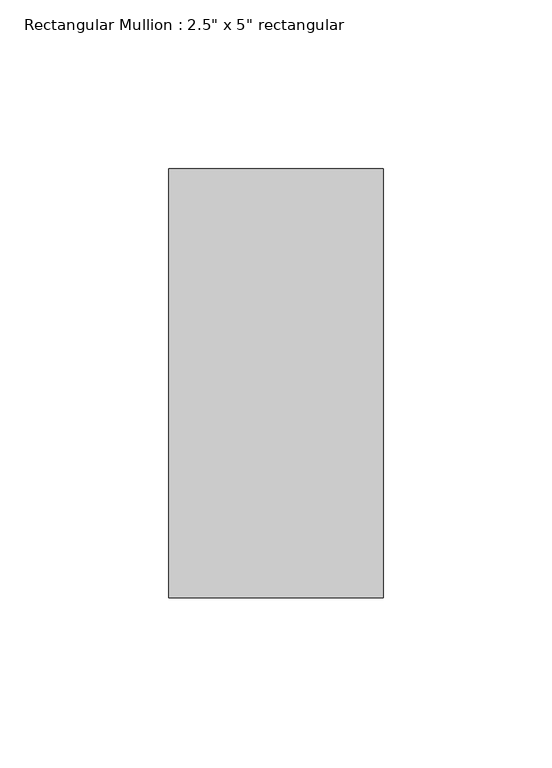
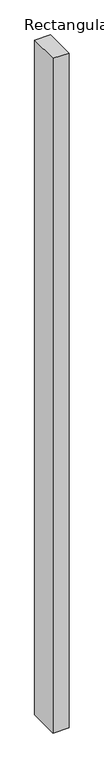
"""IFC4 building model written with IfcOpenShell, lengths in millimetres: member geometry."""

from ifc_helpers import new_model, si_unit, frame, origin, place, context, project, spatial, polyline, outline, extrude, source, transform, mapped, element, save


def member_ae973821(model_context):
    return source(origin(), model_context, "Body", "SweptSolid", [
        extrude(outline(polyline([(31.75, 63.5), (31.75, -63.5), (-31.75, -63.5), (-31.75, 63.5), (31.75, 63.5)])), frame((0.0, 0.0, -2846.788773), z_axis=(0.0, 0.0, 1.0), x_axis=(1.0, 0.0, 0.0)), (0.0, 0.0, 1.0), 2846.788773),
    ])


if __name__ == "__main__":
    model = new_model("IFC4")
    model_context = context("Model", 3, world=origin())
    ifc_project = project(units=[si_unit("LENGTHUNIT", "METRE", prefix="MILLI")], contexts=[model_context])
    site = spatial("IfcSite", under=ifc_project)
    building = spatial("IfcBuilding", under=site)
    placement = place(None, origin())
    member_shape = member_ae973821(model_context)
    element("IfcMember", 1, ObjectType="Rectangular Mullion : 2.5\" x 5\" rectangular", at=placement, inside=building, context=model_context, shape_type="MappedRepresentation", body=[
        mapped(member_shape, transform((0.0, 0.0, 0.0), x_axis=(1.0, 0.0, 0.0), y_axis=(0.0, 1.0, 0.0), z_axis=(0.0, 0.0, 1.0))),
    ])
    save(model, "model.ifc")

# Revit data of these elements
# Type "Rectangular Mullion : 2.5\" x 5\" rectangular"
#   built-in parameter 1007304 = 0.416667 (stored number, unit not read)
#   built-in parameter 1007301 = 0.104167 (stored number, unit not read)
#   built-in parameter 1007300 = 0.104167 (stored number, unit not read)
# Element 1 (IfcMember, "Rectangular Mullion : 2.5\" x 5\" rectangular")
#   Materials on its faces: "Aluminum"
# Materials
#   "Aluminum": class "Metal", colour RGB 247 247 247, transparency 0, Description = "Aluminum 6061", Cost = 0
